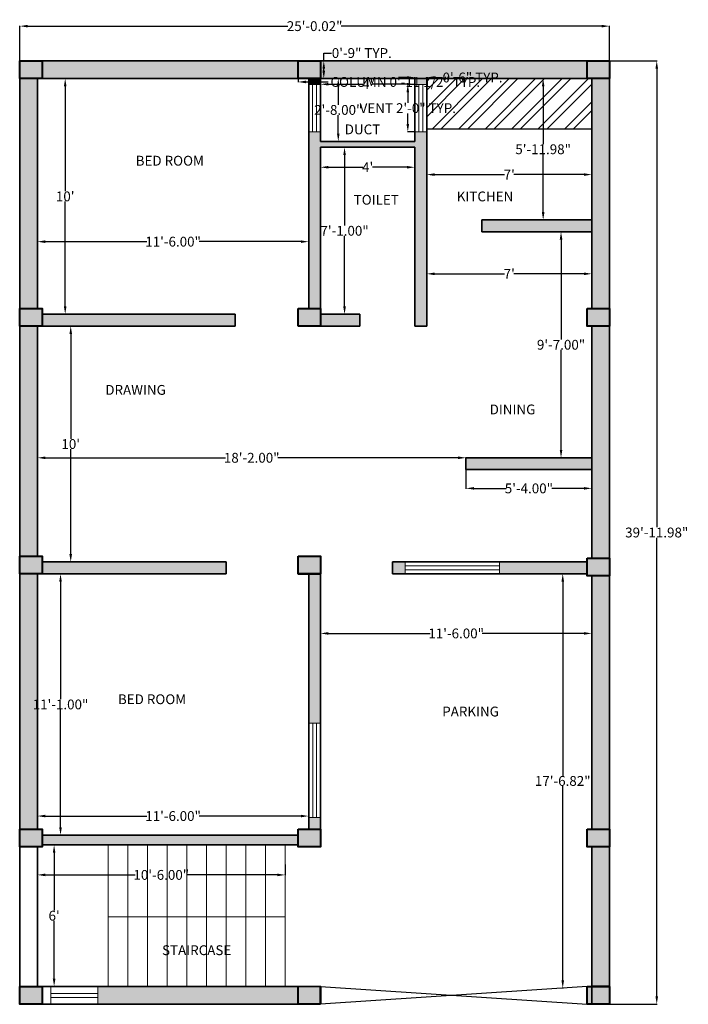
# Model space of a CAD drawing. Units: inches. Extents: x 107756 to 108945, y 133180 to 133782.
# Tile 1 of 3: x 107756 to 108096, y 133257 to 133758. Entities that reach past the tile are written whole.
import ezdxf

# ---------------------------------------------------------------- set-up
doc = ezdxf.new("R2010")
doc.units = ezdxf.units.IN
for name, color, linetype, lineweight in [('A-ANNO-DIMS', 2, 'Continuous', 13), ('A-AREA-IDEN', 7, 'Continuous', 18), ('A-CASE', 8, 'Continuous', 25), ('A-CASE-PATT', 8, 'Continuous', 13), ('A-COLS', 7, 'Continuous', 40), ('A-COLS-PATT', 6, 'Continuous', 13), ('A-DOOR', 3, 'Continuous', 25), ('A-FLOR-STRS', 7, 'Continuous', 18), ('A-GLAZ', 5, 'Continuous', 18), ('A-WALL', 7, 'Continuous', 35), ('A-WALL-PATT', 252, 'Continuous', 13)]:
    doc.layers.add(name, color=color, linetype=linetype, lineweight=lineweight)
doc.styles.get("Standard").update_dxf_attribs({"font": 'arial.ttf', "height": 5})
doc.dimstyles.get("Standard").update_dxf_attribs({"dimtxt": 5, "dimasz": 4, "dimexe": 0.18, "dimexo": 0.0625, "dimgap": 0.09, "dimtad": 0, "dimtih": 1, "dimtoh": 1, "dimzin": 0, "dimdsep": 46, "dimlunit": 3, "dimtxsty": 'Standard', "dimcen": 0.09, "dimclrd": 7, "dimclre": 256, "dimclrt": 256, "dimadec": 0, "dimazin": 0, "dimtfac": 1, "dimtofl": 0, "dimtmove": 0, "dimatfit": 3, "dimfxl": 1, "dimtolj": 1, "dimtzin": 0, "dimarcsym": 0})

# ---------------------------------------------------------------- blocks, each defined once
blk = doc.blocks.new('*D1')
at = {"layer": 'A-ANNO-DIMS', "color": 0, "lineweight": -2, "transparency": 16777216}
for p, q in [((107800.77, 133338.48), (107773.14, 133338.48)), ((107773.32, 133334.48), (107773.32, 133305.12)), ((107773.32, 133270.48), (107773.32, 133299.83)), ((107800.77, 133266.48), (107773.14, 133266.48))]:
    blk.add_line(p, q, dxfattribs=at)
at = {"layer": 'A-ANNO-DIMS', "color": 0, "transparency": 16777216}
for points in [[(107772.65, 133334.48), (107773.99, 133334.48), (107773.32, 133338.48)], [(107772.65, 133270.48), (107773.99, 133270.48), (107773.32, 133266.48)]]:
    blk.add_solid(points, dxfattribs=at)
at = {"layer": 'Defpoints', "color": 0, "transparency": 16777216}
for p in [(107773.32, 133338.48), (107800.84, 133338.48), (107800.84, 133266.48)]:
    blk.add_point(p, dxfattribs=at)
at = {"layer": 'A-ANNO-DIMS', "color": 0, "transparency": 16777216, "insert": (107773.32, 133302.48), "char_height": 5, "attachment_point": 5}
blk.add_mtext("\\A1;6'", dxfattribs=at)
blk = doc.blocks.new('*D2')
at = {"layer": 'A-ANNO-DIMS', "color": 0, "lineweight": -2, "transparency": 16777216}
for p, q in [((107764.84, 133328.53), (107764.84, 133323.07)), ((107890.84, 133328.53), (107890.84, 133323.07)), ((107768.84, 133323.25), (107814.54, 133323.25)), ((107886.84, 133323.25), (107841.13, 133323.25))]:
    blk.add_line(p, q, dxfattribs=at)
at = {"layer": 'A-ANNO-DIMS', "color": 0, "transparency": 16777216}
for points in [[(107768.84, 133323.92), (107768.84, 133322.58), (107764.84, 133323.25)], [(107886.84, 133323.92), (107886.84, 133322.58), (107890.84, 133323.25)]]:
    blk.add_solid(points, dxfattribs=at)
at = {"layer": 'Defpoints', "color": 0, "transparency": 16777216}
for p in [(107764.84, 133328.59), (107890.84, 133328.59), (107890.84, 133323.25)]:
    blk.add_point(p, dxfattribs=at)
at = {"layer": 'A-ANNO-DIMS', "color": 0, "transparency": 16777216, "insert": (107827.84, 133323.25), "char_height": 5, "attachment_point": 5}
blk.add_mtext('\\A1;10\'-6.00"', dxfattribs=at)
blk = doc.blocks.new('*D3')
at = {"layer": 'A-ANNO-DIMS', "color": 0, "lineweight": -2, "transparency": 16777216}
for p, q in [((107764.84, 133357.43), (107764.84, 133353.01)), ((107902.84, 133357.43), (107902.84, 133353.01)), ((107768.84, 133353.19), (107820.54, 133353.19)), ((107898.84, 133353.19), (107847.13, 133353.19))]:
    blk.add_line(p, q, dxfattribs=at)
at = {"layer": 'A-ANNO-DIMS', "color": 0, "transparency": 16777216}
for points in [[(107768.84, 133353.86), (107768.84, 133352.53), (107764.84, 133353.19)], [(107898.84, 133353.86), (107898.84, 133352.53), (107902.84, 133353.19)]]:
    blk.add_solid(points, dxfattribs=at)
at = {"layer": 'Defpoints', "color": 0, "transparency": 16777216}
for p in [(107764.84, 133357.49), (107902.84, 133357.49), (107902.84, 133353.19)]:
    blk.add_point(p, dxfattribs=at)
at = {"layer": 'A-ANNO-DIMS', "color": 0, "transparency": 16777216, "insert": (107833.84, 133353.19), "char_height": 5, "attachment_point": 5}
blk.add_mtext('\\A1;11\'-6.00"', dxfattribs=at)
blk = doc.blocks.new('*D4')
at = {"layer": 'A-ANNO-DIMS', "color": 0, "lineweight": -2, "transparency": 16777216}
for p, q in [((107791.72, 133476.48), (107776.4, 133476.48)), ((107776.58, 133472.48), (107776.58, 133412.62)), ((107776.58, 133347.48), (107776.58, 133407.33)), ((107791.72, 133343.48), (107776.4, 133343.48))]:
    blk.add_line(p, q, dxfattribs=at)
at = {"layer": 'A-ANNO-DIMS', "color": 0, "transparency": 16777216}
for points in [[(107775.91, 133472.48), (107777.24, 133472.48), (107776.58, 133476.48)], [(107775.91, 133347.48), (107777.24, 133347.48), (107776.58, 133343.48)]]:
    blk.add_solid(points, dxfattribs=at)
at = {"layer": 'Defpoints', "color": 0, "transparency": 16777216}
for p in [(107791.78, 133476.48), (107776.58, 133343.48), (107791.78, 133343.48)]:
    blk.add_point(p, dxfattribs=at)
at = {"layer": 'A-ANNO-DIMS', "color": 0, "transparency": 16777216, "insert": (107776.58, 133409.98), "char_height": 5, "attachment_point": 5}
blk.add_mtext('\\A1;11\'-1.00"', dxfattribs=at)
blk = doc.blocks.new('*D5')
at = {"layer": 'A-ANNO-DIMS', "color": 0, "lineweight": -2, "transparency": 16777216}
for p, q in [((107764.84, 133535.52), (107764.84, 133535.3)), ((107768.84, 133535.48), (107860.54, 133535.48)), ((107978.84, 133535.48), (107887.13, 133535.48)), ((107982.84, 133529.54), (107982.84, 133535.66))]:
    blk.add_line(p, q, dxfattribs=at)
at = {"layer": 'A-ANNO-DIMS', "color": 0, "transparency": 16777216}
for points in [[(107768.84, 133536.14), (107768.84, 133534.81), (107764.84, 133535.48)], [(107978.84, 133536.14), (107978.84, 133534.81), (107982.84, 133535.48)]]:
    blk.add_solid(points, dxfattribs=at)
at = {"layer": 'Defpoints', "color": 0, "transparency": 16777216}
for p in [(107764.84, 133535.58), (107982.84, 133535.48), (107982.84, 133529.48)]:
    blk.add_point(p, dxfattribs=at)
at = {"layer": 'A-ANNO-DIMS', "color": 0, "transparency": 16777216, "insert": (107873.84, 133535.48), "char_height": 5, "attachment_point": 5}
blk.add_mtext('\\A1;18\'-2.00"', dxfattribs=at)
blk = doc.blocks.new('*D6')
at = {"layer": 'A-ANNO-DIMS', "color": 0, "lineweight": -2, "transparency": 16777216}
for p, q in [((107775.93, 133602.48), (107781.95, 133602.48)), ((107781.77, 133598.48), (107781.77, 133545.12)), ((107781.77, 133486.48), (107781.77, 133539.83)), ((107775.93, 133482.48), (107781.95, 133482.48))]:
    blk.add_line(p, q, dxfattribs=at)
at = {"layer": 'A-ANNO-DIMS', "color": 0, "transparency": 16777216}
for points in [[(107781.11, 133598.48), (107782.44, 133598.48), (107781.77, 133602.48)], [(107781.11, 133486.48), (107782.44, 133486.48), (107781.77, 133482.48)]]:
    blk.add_solid(points, dxfattribs=at)
at = {"layer": 'Defpoints', "color": 0, "transparency": 16777216}
for p in [(107775.87, 133602.48), (107781.77, 133602.48), (107775.87, 133482.48)]:
    blk.add_point(p, dxfattribs=at)
at = {"layer": 'A-ANNO-DIMS', "color": 0, "transparency": 16777216, "insert": (107781.77, 133542.48), "char_height": 5, "attachment_point": 5}
blk.add_mtext("\\A1;10'", dxfattribs=at)
blk = doc.blocks.new('*D7')
at = {"layer": 'A-ANNO-DIMS', "color": 0, "lineweight": -2, "transparency": 16777216}
for p, q in [((107799.62, 133728.48), (107778.78, 133728.48)), ((107778.96, 133724.48), (107778.96, 133671.12)), ((107778.96, 133612.48), (107778.96, 133665.83)), ((107799.62, 133608.48), (107778.78, 133608.48))]:
    blk.add_line(p, q, dxfattribs=at)
at = {"layer": 'A-ANNO-DIMS', "color": 0, "transparency": 16777216}
for points in [[(107778.29, 133724.48), (107779.62, 133724.48), (107778.96, 133728.48)], [(107778.29, 133612.48), (107779.62, 133612.48), (107778.96, 133608.48)]]:
    blk.add_solid(points, dxfattribs=at)
at = {"layer": 'Defpoints', "color": 0, "transparency": 16777216}
for p in [(107778.96, 133728.48), (107799.68, 133728.48), (107799.68, 133608.48)]:
    blk.add_point(p, dxfattribs=at)
at = {"layer": 'A-ANNO-DIMS', "color": 0, "transparency": 16777216, "insert": (107778.96, 133668.48), "char_height": 5, "attachment_point": 5}
blk.add_mtext("\\A1;10'", dxfattribs=at)
blk = doc.blocks.new('*D8')
at = {"layer": 'A-ANNO-DIMS', "color": 0, "lineweight": -2, "transparency": 16777216}
for p, q in [((107764.84, 133651.21), (107764.84, 133645.27)), ((107902.84, 133651.21), (107902.84, 133645.27)), ((107768.84, 133645.45), (107820.54, 133645.45)), ((107898.84, 133645.45), (107847.13, 133645.45))]:
    blk.add_line(p, q, dxfattribs=at)
at = {"layer": 'A-ANNO-DIMS', "color": 0, "transparency": 16777216}
for points in [[(107768.84, 133646.11), (107768.84, 133644.78), (107764.84, 133645.45)], [(107898.84, 133646.11), (107898.84, 133644.78), (107902.84, 133645.45)]]:
    blk.add_solid(points, dxfattribs=at)
at = {"layer": 'Defpoints', "color": 0, "transparency": 16777216}
for p in [(107764.84, 133651.27), (107902.84, 133651.27), (107902.84, 133645.45)]:
    blk.add_point(p, dxfattribs=at)
at = {"layer": 'A-ANNO-DIMS', "color": 0, "transparency": 16777216, "insert": (107833.84, 133645.45), "char_height": 5, "attachment_point": 5}
blk.add_mtext('\\A1;11\'-6.00"', dxfattribs=at)
blk = doc.blocks.new('*D9')
at = {"layer": 'A-ANNO-DIMS', "color": 0, "lineweight": -2, "transparency": 16777216}
for p, q in [((107908.84, 133726.32), (107908.84, 133725.36)), ((107912.84, 133725.54), (107930.35, 133725.54)), ((107952.84, 133725.54), (107935.33, 133725.54)), ((107956.84, 133726.32), (107956.84, 133725.36))]:
    blk.add_line(p, q, dxfattribs=at)
at = {"layer": 'A-ANNO-DIMS', "color": 0, "transparency": 16777216}
for points in [[(107912.84, 133726.21), (107912.84, 133724.88), (107908.84, 133725.54)], [(107952.84, 133726.21), (107952.84, 133724.88), (107956.84, 133725.54)]]:
    blk.add_solid(points, dxfattribs=at)
at = {"layer": 'Defpoints', "color": 0, "transparency": 16777216}
for p in [(107908.84, 133726.38), (107956.84, 133726.38), (107956.84, 133725.54)]:
    blk.add_point(p, dxfattribs=at)
at = {"layer": 'A-ANNO-DIMS', "color": 0, "transparency": 16777216, "insert": (107932.84, 133725.54), "char_height": 5, "attachment_point": 5}
blk.add_mtext("\\A1;4'", dxfattribs=at)
blk = doc.blocks.new('*D10')
at = {"layer": 'A-ANNO-DIMS', "color": 0, "lineweight": -2, "transparency": 16777216}
for p, q in [((107914.64, 133728.48), (107918.05, 133728.48)), ((107917.87, 133724.48), (107917.87, 133715.12)), ((107917.87, 133700.48), (107917.87, 133709.83)), ((107914.64, 133696.48), (107918.05, 133696.48))]:
    blk.add_line(p, q, dxfattribs=at)
at = {"layer": 'A-ANNO-DIMS', "color": 0, "transparency": 16777216}
for points in [[(107917.2, 133724.48), (107918.54, 133724.48), (107917.87, 133728.48)], [(107917.2, 133700.48), (107918.54, 133700.48), (107917.87, 133696.48)]]:
    blk.add_solid(points, dxfattribs=at)
at = {"layer": 'Defpoints', "color": 0, "transparency": 16777216}
for p in [(107914.57, 133728.48), (107917.87, 133728.48), (107914.57, 133696.48)]:
    blk.add_point(p, dxfattribs=at)
at = {"layer": 'A-ANNO-DIMS', "color": 0, "transparency": 16777216, "insert": (107917.87, 133712.48), "char_height": 5, "attachment_point": 5}
blk.add_mtext('\\A1;2\'-8.00"', dxfattribs=at)
blk = doc.blocks.new('*D11')
at = {"layer": 'A-ANNO-DIMS', "color": 0, "lineweight": -2, "transparency": 16777216}
for p, q in [((107922.84, 133693.48), (107920.89, 133693.48)), ((107921.07, 133689.48), (107921.07, 133653.62)), ((107921.07, 133612.48), (107921.07, 133648.33)), ((107922.84, 133608.48), (107920.89, 133608.48))]:
    blk.add_line(p, q, dxfattribs=at)
at = {"layer": 'A-ANNO-DIMS', "color": 0, "transparency": 16777216}
for points in [[(107920.41, 133689.48), (107921.74, 133689.48), (107921.07, 133693.48)], [(107920.41, 133612.48), (107921.74, 133612.48), (107921.07, 133608.48)]]:
    blk.add_solid(points, dxfattribs=at)
at = {"layer": 'Defpoints', "color": 0, "transparency": 16777216}
for p in [(107921.07, 133693.48), (107922.9, 133693.48), (107922.9, 133608.48)]:
    blk.add_point(p, dxfattribs=at)
at = {"layer": 'A-ANNO-DIMS', "color": 0, "transparency": 16777216, "insert": (107921.07, 133650.98), "char_height": 5, "attachment_point": 5}
blk.add_mtext('\\A1;7\'-1.00"', dxfattribs=at)
blk = doc.blocks.new('*D12')
at = {"layer": 'A-ANNO-DIMS', "color": 0, "lineweight": -2, "transparency": 16777216}
for p, q in [((107908.84, 133693.41), (107908.84, 133683.14)), ((107956.84, 133693.41), (107956.84, 133683.14)), ((107912.84, 133683.32), (107930.35, 133683.32)), ((107952.84, 133683.32), (107935.33, 133683.32))]:
    blk.add_line(p, q, dxfattribs=at)
at = {"layer": 'A-ANNO-DIMS', "color": 0, "transparency": 16777216}
for points in [[(107912.84, 133683.98), (107912.84, 133682.65), (107908.84, 133683.32)], [(107952.84, 133683.98), (107952.84, 133682.65), (107956.84, 133683.32)]]:
    blk.add_solid(points, dxfattribs=at)
at = {"layer": 'Defpoints', "color": 0, "transparency": 16777216}
for p in [(107908.84, 133693.48), (107956.84, 133693.48), (107908.84, 133683.32)]:
    blk.add_point(p, dxfattribs=at)
at = {"layer": 'A-ANNO-DIMS', "color": 0, "transparency": 16777216, "insert": (107932.84, 133683.32), "char_height": 5, "attachment_point": 5}
blk.add_mtext("\\A1;4'", dxfattribs=at)
blk = doc.blocks.new('*D13')
at = {"layer": 'A-ANNO-DIMS', "color": 0, "lineweight": -2, "transparency": 16777216}
for p, q in [((108046.77, 133728.45), (108021.91, 133728.45)), ((108022.09, 133724.45), (108022.09, 133695.11)), ((108022.09, 133660.48), (108022.09, 133689.82)), ((108046.77, 133656.48), (108021.91, 133656.48))]:
    blk.add_line(p, q, dxfattribs=at)
at = {"layer": 'A-ANNO-DIMS', "color": 0, "transparency": 16777216}
for points in [[(108021.43, 133724.45), (108022.76, 133724.45), (108022.09, 133728.45)], [(108021.43, 133660.48), (108022.76, 133660.48), (108022.09, 133656.48)]]:
    blk.add_solid(points, dxfattribs=at)
at = {"layer": 'Defpoints', "color": 0, "transparency": 16777216}
for p in [(108022.09, 133728.45), (108046.84, 133728.45), (108046.84, 133656.48)]:
    blk.add_point(p, dxfattribs=at)
at = {"layer": 'A-ANNO-DIMS', "color": 0, "transparency": 16777216, "insert": (108022.09, 133692.46), "char_height": 5, "attachment_point": 5}
blk.add_mtext('\\A1;5\'-11.98"', dxfattribs=at)
blk = doc.blocks.new('*D14')
at = {"layer": 'A-ANNO-DIMS', "color": 0, "lineweight": -2, "transparency": 16777216}
for p, q in [((107962.84, 133691.71), (107962.84, 133679.39)), ((108046.84, 133691.71), (108046.84, 133679.39)), ((107966.84, 133679.57), (108002.47, 133679.57)), ((108042.84, 133679.57), (108007.21, 133679.57))]:
    blk.add_line(p, q, dxfattribs=at)
at = {"layer": 'A-ANNO-DIMS', "color": 0, "transparency": 16777216}
for points in [[(107966.84, 133680.24), (107966.84, 133678.91), (107962.84, 133679.57)], [(108042.84, 133680.24), (108042.84, 133678.91), (108046.84, 133679.57)]]:
    blk.add_solid(points, dxfattribs=at)
at = {"layer": 'Defpoints', "color": 0, "transparency": 16777216}
for p in [(107962.84, 133691.78), (108046.84, 133691.78), (108046.84, 133679.57)]:
    blk.add_point(p, dxfattribs=at)
at = {"layer": 'A-ANNO-DIMS', "color": 0, "transparency": 16777216, "insert": (108004.84, 133679.57), "char_height": 5, "attachment_point": 5}
blk.add_mtext("\\A1;7'", dxfattribs=at)
blk = doc.blocks.new('*D15')
at = {"layer": 'A-ANNO-DIMS', "color": 0, "lineweight": -2, "transparency": 16777216}
for p, q in [((107962.84, 133629.16), (107962.84, 133628.9)), ((107966.84, 133629.08), (108002.47, 133629.08)), ((108042.84, 133629.08), (108007.21, 133629.08)), ((108046.84, 133629.16), (108046.84, 133628.9))]:
    blk.add_line(p, q, dxfattribs=at)
at = {"layer": 'A-ANNO-DIMS', "color": 0, "transparency": 16777216}
for points in [[(107966.84, 133629.75), (107966.84, 133628.42), (107962.84, 133629.08)], [(108042.84, 133629.75), (108042.84, 133628.42), (108046.84, 133629.08)]]:
    blk.add_solid(points, dxfattribs=at)
at = {"layer": 'Defpoints', "color": 0, "transparency": 16777216}
for p in [(107962.84, 133629.23), (107962.84, 133629.08), (108046.84, 133629.23)]:
    blk.add_point(p, dxfattribs=at)
at = {"layer": 'A-ANNO-DIMS', "color": 0, "transparency": 16777216, "insert": (108004.84, 133629.08), "char_height": 5, "attachment_point": 5}
blk.add_mtext("\\A1;7'", dxfattribs=at)
blk = doc.blocks.new('*D16')
at = {"layer": 'A-ANNO-DIMS', "color": 0, "lineweight": -2, "transparency": 16777216}
for p, q in [((108037.82, 133650.48), (108031.01, 133650.48)), ((108031.19, 133646.48), (108031.19, 133595.62)), ((108031.19, 133539.48), (108031.19, 133590.33)), ((108037.82, 133535.48), (108031.01, 133535.48))]:
    blk.add_line(p, q, dxfattribs=at)
at = {"layer": 'A-ANNO-DIMS', "color": 0, "transparency": 16777216}
for points in [[(108030.53, 133646.48), (108031.86, 133646.48), (108031.19, 133650.48)], [(108030.53, 133539.48), (108031.86, 133539.48), (108031.19, 133535.48)]]:
    blk.add_solid(points, dxfattribs=at)
at = {"layer": 'Defpoints', "color": 0, "transparency": 16777216}
for p in [(108037.89, 133650.48), (108031.19, 133535.48), (108037.89, 133535.48)]:
    blk.add_point(p, dxfattribs=at)
at = {"layer": 'A-ANNO-DIMS', "color": 0, "transparency": 16777216, "insert": (108031.19, 133592.98), "char_height": 5, "attachment_point": 5}
blk.add_mtext('\\A1;9\'-7.00"', dxfattribs=at)
blk = doc.blocks.new('*D17')
at = {"layer": 'A-ANNO-DIMS', "color": 0, "lineweight": -2, "transparency": 16777216}
for p, q in [((107982.84, 133529.41), (107982.84, 133519.74)), ((108046.84, 133529.41), (108046.84, 133519.74)), ((107986.84, 133519.92), (108003.25, 133519.92)), ((108042.84, 133519.92), (108026.43, 133519.92))]:
    blk.add_line(p, q, dxfattribs=at)
at = {"layer": 'A-ANNO-DIMS', "color": 0, "transparency": 16777216}
for points in [[(107986.84, 133520.59), (107986.84, 133519.26), (107982.84, 133519.92)], [(108042.84, 133520.59), (108042.84, 133519.26), (108046.84, 133519.92)]]:
    blk.add_solid(points, dxfattribs=at)
at = {"layer": 'Defpoints', "color": 0, "transparency": 16777216}
for p in [(107982.84, 133529.48), (108046.84, 133529.48), (107982.84, 133519.92)]:
    blk.add_point(p, dxfattribs=at)
at = {"layer": 'A-ANNO-DIMS', "color": 0, "transparency": 16777216, "insert": (108014.84, 133519.92), "char_height": 5, "attachment_point": 5}
blk.add_mtext('\\A1;5\'-4.00"', dxfattribs=at)
blk = doc.blocks.new('*D18')
at = {"layer": 'A-ANNO-DIMS', "color": 0, "lineweight": -2, "transparency": 16777216}
for p, q in [((107908.84, 133439.92), (107908.84, 133446.29)), ((107912.84, 133446.11), (107964.54, 133446.11)), ((108042.84, 133446.11), (107991.13, 133446.11)), ((108046.84, 133439.92), (108046.84, 133446.29))]:
    blk.add_line(p, q, dxfattribs=at)
at = {"layer": 'A-ANNO-DIMS', "color": 0, "transparency": 16777216}
for points in [[(107912.84, 133446.78), (107912.84, 133445.45), (107908.84, 133446.11)], [(108042.84, 133446.78), (108042.84, 133445.45), (108046.84, 133446.11)]]:
    blk.add_solid(points, dxfattribs=at)
at = {"layer": 'Defpoints', "color": 0, "transparency": 16777216}
for p in [(107908.84, 133446.11), (107908.84, 133439.86), (108046.84, 133439.86)]:
    blk.add_point(p, dxfattribs=at)
at = {"layer": 'A-ANNO-DIMS', "color": 0, "transparency": 16777216, "insert": (107977.84, 133446.11), "char_height": 5, "attachment_point": 5}
blk.add_mtext('\\A1;11\'-6.00"', dxfattribs=at)
blk = doc.blocks.new('*D19')
at = {"layer": 'A-ANNO-DIMS', "color": 0, "lineweight": -2, "transparency": 16777216}
for p, q in [((108055.86, 133737.45), (108080.05, 133737.45)), ((108079.87, 133733.45), (108079.87, 133500.11)), ((108079.87, 133261.48), (108079.87, 133494.82)), ((108055.9, 133257.48), (108080.05, 133257.48))]:
    blk.add_line(p, q, dxfattribs=at)
at = {"layer": 'A-ANNO-DIMS', "color": 0, "transparency": 16777216}
for points in [[(108079.21, 133733.45), (108080.54, 133733.45), (108079.87, 133737.45)], [(108079.21, 133261.48), (108080.54, 133261.48), (108079.87, 133257.48)]]:
    blk.add_solid(points, dxfattribs=at)
at = {"layer": 'Defpoints', "color": 0, "transparency": 16777216}
for p in [(108055.8, 133737.45), (108055.84, 133257.48), (108079.87, 133257.48)]:
    blk.add_point(p, dxfattribs=at)
at = {"layer": 'A-ANNO-DIMS', "color": 0, "transparency": 16777216, "insert": (108079.87, 133497.46), "char_height": 5, "attachment_point": 5}
blk.add_mtext('\\A1;39\'-11.98"', dxfattribs=at)
blk = doc.blocks.new('*D20')
at = {"layer": 'A-ANNO-DIMS', "color": 0, "lineweight": -2, "transparency": 16777216}
for p, q in [((107755.84, 133737.54), (107755.84, 133755.29)), ((107759.84, 133755.11), (107892.27, 133755.11)), ((108051.86, 133755.11), (107919.42, 133755.11)), ((108055.86, 133737.51), (108055.86, 133755.29))]:
    blk.add_line(p, q, dxfattribs=at)
at = {"layer": 'A-ANNO-DIMS', "color": 0, "transparency": 16777216}
for points in [[(107759.84, 133755.77), (107759.84, 133754.44), (107755.84, 133755.11)], [(108051.86, 133755.77), (108051.86, 133754.44), (108055.86, 133755.11)]]:
    blk.add_solid(points, dxfattribs=at)
at = {"layer": 'Defpoints', "color": 0, "transparency": 16777216}
for p in [(108055.86, 133755.11), (107755.84, 133737.48), (108055.86, 133737.45)]:
    blk.add_point(p, dxfattribs=at)
at = {"layer": 'A-ANNO-DIMS', "color": 0, "transparency": 16777216, "insert": (107905.85, 133755.11), "char_height": 5, "attachment_point": 5}
blk.add_mtext('\\A1;25\'-0.02"', dxfattribs=at)
blk = doc.blocks.new('*D21')
at = {"layer": 'A-ANNO-DIMS', "color": 0, "lineweight": -2, "transparency": 16777216}
for p, q in [((108031.38, 133476.48), (108032.23, 133476.48)), ((108032.05, 133472.48), (108032.05, 133373.71)), ((108032.05, 133269.65), (108032.05, 133368.42)), ((108032.12, 133265.65), (108032.23, 133265.65))]:
    blk.add_line(p, q, dxfattribs=at)
at = {"layer": 'A-ANNO-DIMS', "color": 0, "transparency": 16777216}
for points in [[(108031.39, 133472.48), (108032.72, 133472.48), (108032.05, 133476.48)], [(108031.39, 133269.65), (108032.72, 133269.65), (108032.05, 133265.65)]]:
    blk.add_solid(points, dxfattribs=at)
at = {"layer": 'Defpoints', "color": 0, "transparency": 16777216}
for p in [(108031.32, 133476.48), (108032.05, 133265.65), (108032.05, 133265.65)]:
    blk.add_point(p, dxfattribs=at)
at = {"layer": 'A-ANNO-DIMS', "color": 0, "transparency": 16777216, "insert": (108032.05, 133371.06), "char_height": 5, "attachment_point": 5}
blk.add_mtext('\\A1;17\'-6.82"', dxfattribs=at)
blk = doc.blocks.new('WIN-VENT-24IN')
for p, q in [((0, 24), (6, 24)), ((2, 0), (2, 24)), ((4, 0), (4, 24)), ((0, 0), (6, 0))]:
    blk.add_line(p, q)
blk = doc.blocks.new('COL-RECT-11_37x9')
blk.add_lwpolyline([(0, 9), (11.37, 9), (11.37, 0), (0, 0)], close=True)
blk = doc.blocks.new('*D45')
at = {"layer": 'A-ANNO-DIMS', "lineweight": -2, "transparency": 16777216}
for p, q in [((107897.42, 133728.36), (107897.42, 133726.53)), ((107908.8, 133728.36), (107908.8, 133726.53))]:
    blk.add_line(p, q, dxfattribs=at)
at = {"layer": 'A-ANNO-DIMS', "color": 7, "lineweight": -2, "transparency": 16777216}
for p, q in [((107901.42, 133726.71), (107904.8, 133726.71)), ((107908.8, 133726.71), (107912.8, 133726.71))]:
    blk.add_line(p, q, dxfattribs=at)
at = {"layer": 'A-ANNO-DIMS', "color": 7, "transparency": 16777216}
for points in [[(107901.42, 133727.38), (107901.42, 133726.05), (107897.42, 133726.71)], [(107904.8, 133727.38), (107904.8, 133726.05), (107908.8, 133726.71)]]:
    blk.add_solid(points, dxfattribs=at)
at = {"layer": 'Defpoints', "color": 0, "transparency": 16777216}
for p in [(107897.42, 133728.42), (107908.8, 133728.42), (107908.8, 133726.71)]:
    blk.add_point(p, dxfattribs=at)
at = {"layer": 'A-ANNO-DIMS', "transparency": 16777216, "insert": (107951.97, 133726.71), "char_height": 5, "attachment_point": 5}
blk.add_mtext('\\A1;COLUMN 0\'-11 1/2" TYP.', dxfattribs=at)
blk = doc.blocks.new('*D46')
at = {"layer": 'A-ANNO-DIMS', "lineweight": -2, "transparency": 16777216}
for p, q in [((107908.86, 133737.42), (107910.68, 133737.42)), ((107908.86, 133728.42), (107910.68, 133728.42))]:
    blk.add_line(p, q, dxfattribs=at)
at = {"layer": 'A-ANNO-DIMS', "color": 7, "lineweight": -2, "transparency": 16777216}
for p, q in [((107910.5, 133737.42), (107910.5, 133741.42)), ((107910.5, 133741.42), (107914.5, 133741.42)), ((107910.5, 133732.42), (107910.5, 133733.42))]:
    blk.add_line(p, q, dxfattribs=at)
at = {"layer": 'A-ANNO-DIMS', "color": 7, "transparency": 16777216}
for points in [[(107909.83, 133733.42), (107911.17, 133733.42), (107910.5, 133737.42)], [(107909.83, 133732.42), (107911.17, 133732.42), (107910.5, 133728.42)]]:
    blk.add_solid(points, dxfattribs=at)
at = {"layer": 'Defpoints', "color": 0, "transparency": 16777216}
for p in [(107908.8, 133737.42), (107910.5, 133737.42), (107908.8, 133728.42)]:
    blk.add_point(p, dxfattribs=at)
at = {"layer": 'A-ANNO-DIMS', "transparency": 16777216, "insert": (107929.83, 133741.42), "char_height": 5, "attachment_point": 5}
blk.add_mtext('\\A1;0\'-9" TYP.', dxfattribs=at)
blk = doc.blocks.new('*D47')
at = {"layer": 'A-ANNO-DIMS', "lineweight": -2, "transparency": 16777216}
for p, q in [((107956.77, 133725.38), (107953.06, 133725.38)), ((107956.77, 133701.38), (107953.06, 133701.38))]:
    blk.add_line(p, q, dxfattribs=at)
at = {"layer": 'A-ANNO-DIMS', "color": 7, "lineweight": -2, "transparency": 16777216}
for p, q in [((107953.24, 133721.38), (107953.24, 133716.02)), ((107953.24, 133705.38), (107953.24, 133710.73))]:
    blk.add_line(p, q, dxfattribs=at)
at = {"layer": 'A-ANNO-DIMS', "color": 7, "transparency": 16777216}
for points in [[(107952.57, 133721.38), (107953.9, 133721.38), (107953.24, 133725.38)], [(107952.57, 133705.38), (107953.9, 133705.38), (107953.24, 133701.38)]]:
    blk.add_solid(points, dxfattribs=at)
at = {"layer": 'Defpoints', "color": 0, "transparency": 16777216}
for p in [(107953.24, 133725.38), (107956.84, 133725.38), (107956.84, 133701.38)]:
    blk.add_point(p, dxfattribs=at)
at = {"layer": 'A-ANNO-DIMS', "transparency": 16777216, "insert": (107953.24, 133713.38), "char_height": 5, "attachment_point": 5}
blk.add_mtext('\\A1;VENT 2\'-0" TYP.', dxfattribs=at)
blk = doc.blocks.new('*D48')
at = {"layer": 'A-ANNO-DIMS', "color": 7, "lineweight": -2, "transparency": 16777216}
for p, q in [((107952.84, 133728.98), (107948.84, 133728.98)), ((107966.84, 133728.98), (107970.84, 133728.98))]:
    blk.add_line(p, q, dxfattribs=at)
at = {"layer": 'A-ANNO-DIMS', "lineweight": -2, "transparency": 16777216}
for p, q in [((107956.84, 133725.44), (107956.84, 133729.16)), ((107962.84, 133725.44), (107962.84, 133729.16))]:
    blk.add_line(p, q, dxfattribs=at)
at = {"layer": 'A-ANNO-DIMS', "color": 7, "transparency": 16777216}
for points in [[(107952.84, 133729.64), (107952.84, 133728.31), (107956.84, 133728.98)], [(107966.84, 133729.64), (107966.84, 133728.31), (107962.84, 133728.98)]]:
    blk.add_solid(points, dxfattribs=at)
at = {"layer": 'Defpoints', "color": 0, "transparency": 16777216}
for p in [(107962.84, 133728.98), (107956.84, 133725.38), (107962.84, 133725.38)]:
    blk.add_point(p, dxfattribs=at)
at = {"layer": 'A-ANNO-DIMS', "transparency": 16777216, "insert": (107986.17, 133728.98), "char_height": 5, "attachment_point": 5}
blk.add_mtext('\\A1;0\'-6" TYP.', dxfattribs=at)

msp = doc.modelspace()

# ---------------------------------------------------------------- hatches: boundary and pattern name
at = {"layer": 'A-CASE-PATT'}
h = msp.add_hatch(dxfattribs=at)
h.set_pattern_fill('ANSI32', color=256)
h.set_pattern_definition([(45, (717.227, 52.435), (-6.7351921, 6.7351921), []), (45, (721.718, 52.435), (-6.7351921, 6.7351921), [])])
h.paths.add_polyline_path([(108046.837, 133702.908), (108046.837, 133728.452), (108044.427, 133728.452), (107962.837, 133728.459), (107962.837, 133702.908)])
at = {"layer": 'A-COLS-PATT'}
h = msp.add_hatch(color=256, dxfattribs=at)
h.dxf.hatch_style = 1
h.paths.add_polyline_path([(107767.208, 133485.477), (107755.837, 133485.477), (107755.837, 133476.477), (107767.208, 133476.477)])
h.paths.add_polyline_path([(107908.837, 133485.477), (107897.467, 133485.477), (107897.467, 133476.477), (107908.837, 133476.477)])
h.paths.add_polyline_path([(107908.837, 133346.477), (107897.467, 133346.477), (107897.467, 133337.477), (107908.837, 133337.477)])
h.paths.add_polyline_path([(107767.208, 133346.477), (107755.837, 133346.477), (107755.837, 133337.477), (107767.208, 133337.477)])
h.paths.add_polyline_path([(107767.208, 133266.477), (107755.837, 133266.477), (107755.837, 133257.477), (107767.208, 133257.477)])
h.paths.add_polyline_path([(107908.837, 133266.477), (107897.467, 133266.477), (107897.467, 133257.477), (107908.837, 133257.477)])
h.paths.add_polyline_path([(108055.837, 133266.477), (108046.837, 133266.477), (108046.837, 133257.477), (108055.837, 133257.477)])
h.paths.add_polyline_path([(108046.837, 133266.477), (108044.467, 133266.477), (108044.467, 133257.477), (108046.837, 133257.477)])
h.paths.add_polyline_path([(108055.837, 133346.477), (108044.467, 133346.477), (108044.467, 133337.477), (108055.837, 133337.477)])
h.paths.add_polyline_path([(108055.837, 133484.477), (108044.467, 133484.477), (108044.467, 133475.477), (108055.837, 133475.477)])
h.paths.add_polyline_path([(108055.837, 133611.477), (108044.467, 133611.477), (108044.467, 133602.477), (108055.837, 133602.477)])
h.paths.add_polyline_path([(108055.798, 133737.452), (108044.427, 133737.452), (108044.427, 133728.477), (108046.837, 133728.477), (108055.798, 133728.452)])
h.paths.add_polyline_path([(107767.208, 133737.477), (107755.837, 133737.477), (107755.837, 133728.477), (107767.208, 133728.477)])
h.paths.add_polyline_path([(107908.795, 133737.42), (107897.425, 133737.42), (107897.425, 133728.477), (107908.795, 133728.477)])
h.paths.add_polyline_path([(107908.837, 133611.477), (107897.467, 133611.477), (107897.467, 133602.477), (107908.837, 133602.477)])
h.paths.add_polyline_path([(107767.184, 133611.478), (107755.837, 133611.478), (107755.837, 133602.478), (107767.184, 133602.478)])
at = {"layer": 'A-WALL-PATT'}
h = msp.add_hatch(color=256, dxfattribs=at)
h.dxf.hatch_style = 1
h.paths.add_polyline_path([(107764.837, 133476.477), (107755.837, 133476.477), (107755.837, 133346.477), (107764.837, 133346.477)])
h.paths.add_polyline_path([(107860.893, 133476.477), (107860.893, 133482.477), (107767.208, 133482.477), (107767.208, 133476.477)])
h.paths.add_polyline_path([(107897.467, 133338.477), (107897.467, 133343.477), (107767.208, 133343.477), (107767.208, 133338.477)])
h.paths.add_polyline_path([(107908.837, 133476.477), (107902.837, 133476.477), (107902.837, 133400.531), (107908.837, 133400.531)])
h.paths.add_polyline_path([(107908.837, 133346.477), (107908.837, 133352.531), (107902.837, 133352.531), (107902.837, 133346.477)])
h.paths.add_polyline_path([(107999.961, 133482.477), (107999.961, 133476.477), (108044.467, 133476.477), (108044.467, 133482.477)])
h.paths.add_polyline_path([(107945.411, 133482.477), (107945.411, 133476.477), (107951.961, 133476.477), (107951.961, 133482.477)])
h.paths.add_polyline_path([(107982.837, 133535.477), (107982.837, 133529.477), (108046.837, 133529.477), (108046.837, 133535.477)])
h.paths.add_polyline_path([(108046.837, 133529.477), (108046.837, 133484.477), (108055.837, 133484.477), (108055.837, 133602.477), (108046.837, 133602.477)])
h.paths.add_polyline_path([(108055.837, 133475.477), (108046.837, 133475.477), (108046.837, 133346.477), (108055.837, 133346.477)])
h.paths.add_polyline_path([(108055.837, 133337.477), (108046.837, 133337.477), (108046.837, 133266.477), (108055.837, 133266.477)])
h.paths.add_polyline_path([(108046.837, 133611.477), (108055.837, 133611.477), (108055.837, 133728.452), (108046.837, 133728.452)])
h.paths.add_polyline_path([(107956.837, 133608.477), (107956.837, 133602.477), (107962.837, 133602.477), (107962.837, 133701.376), (107956.837, 133701.376), (107956.837, 133696.477), (107908.837, 133696.477), (107908.837, 133701.376), (107902.837, 133701.376), (107902.837, 133611.477), (107908.837, 133611.477), (107908.837, 133693.477), (107956.837, 133693.477)])
h.paths.add_polyline_path([(107962.837, 133725.376), (107962.837, 133728.477), (107956.837, 133728.477), (107956.837, 133725.376)])
h.paths.add_polyline_path([(108044.427, 133728.477), (108044.427, 133737.477), (107908.837, 133737.477), (107908.837, 133728.477)])
h.paths.add_polyline_path([(107767.208, 133737.477), (107767.208, 133728.477), (107897.425, 133728.477), (107897.425, 133737.477)])
h.paths.add_polyline_path([(107764.837, 133728.477), (107755.837, 133728.477), (107755.837, 133611.478), (107764.837, 133611.478)])
h.paths.add_polyline_path([(107755.837, 133485.477), (107764.837, 133485.477), (107764.837, 133602.478), (107755.837, 133602.478)])
h.paths.add_polyline_path([(107795.626, 133266.477), (107795.626, 133257.477), (107897.467, 133257.477), (107897.467, 133266.477)])
h = msp.add_hatch(color=256, dxfattribs=at)
h.dxf.hatch_style = 1
h.paths.add_polyline_path([(107902.837, 133728.42), (107902.837, 133725.376), (107908.837, 133725.376), (107908.837, 133728.42)])
h = msp.add_hatch(color=256, dxfattribs=at)
h.dxf.hatch_style = 1
h.paths.add_polyline_path([(108046.837, 133650.477), (108046.837, 133656.477), (107990.837, 133656.477), (107990.837, 133650.477)])
h = msp.add_hatch(color=256, dxfattribs=at)
h.dxf.hatch_style = 1
h.paths.add_polyline_path([(107865.467, 133608.477), (107767.184, 133608.477), (107767.184, 133602.477), (107865.467, 133602.477)])
h.paths.add_polyline_path([(107908.837, 133608.477), (107908.837, 133602.477), (107928.837, 133602.477), (107928.837, 133608.477)])

# ---------------------------------------------------------------- linework, layer by layer
at = {"layer": 'A-CASE'}
msp.add_line((107962.837, 133702.908), (108046.837, 133702.908), dxfattribs=at)
at = {"layer": 'A-COLS'}
for p, q in [((107897.467, 133611.477), (107908.837, 133611.477)), ((107897.467, 133602.477), (107897.467, 133611.477)), ((107908.837, 133611.477), (107908.837, 133602.477)), ((107908.837, 133602.477), (107897.467, 133602.477)), ((107897.467, 133476.477), (107908.837, 133476.477)), ((107897.467, 133257.477), (107897.467, 133266.477)), ((107908.837, 133266.477), (107908.837, 133257.477)), ((107908.837, 133257.477), (107897.467, 133257.477))]:
    msp.add_line(p, q, dxfattribs=at)
msp.add_lwpolyline([(107908.837, 133257.477), (107908.837, 133257.477), (107908.837, 133266.477), (107908.837, 133266.477)], close=True, dxfattribs=at)
msp.add_lwpolyline([(107908.837, 133257.477), (107908.837, 133257.477), (107908.837, 133266.477), (107908.837, 133266.477)], close=True, dxfattribs=at)
for points in [[(108055.837, 133266.477), (108046.837, 133266.477)], [(108055.837, 133257.477), (108046.837, 133257.477)]]:
    msp.add_lwpolyline(points, dxfattribs=at)
at = {"layer": 'A-DOOR'}
for p, q in [((107908.837, 133266.477), (108044.467, 133257.477)), ((108044.467, 133266.477), (107908.837, 133257.477))]:
    msp.add_line(p, q, dxfattribs=at)
at = {"layer": 'A-FLOR-STRS'}
for p, q in [((107800.837, 133266.477), (107800.837, 133338.477)), ((107810.837, 133266.477), (107810.837, 133338.477)), ((107820.837, 133266.477), (107820.837, 133338.477)), ((107830.837, 133266.477), (107830.837, 133338.477)), ((107840.837, 133266.477), (107840.837, 133338.477)), ((107850.837, 133266.477), (107850.837, 133338.477)), ((107860.837, 133266.477), (107860.837, 133338.477)), ((107870.837, 133266.477), (107870.837, 133338.477)), ((107880.837, 133266.477), (107880.837, 133338.477)), ((107890.837, 133266.477), (107890.837, 133338.477)), ((107800.837, 133301.977), (107890.837, 133301.977))]:
    msp.add_line(p, q, dxfattribs=at)
at = {"layer": 'A-GLAZ'}
for p, q in [((107951.961, 133482.477), (107951.961, 133476.477)), ((107999.961, 133482.477), (107999.961, 133476.477)), ((107999.961, 133480.477), (107951.961, 133480.477)), ((107999.961, 133478.477), (107951.961, 133478.477)), ((107908.87, 133400.531), (107902.837, 133400.531)), ((107904.854, 133352.531), (107904.854, 133400.531)), ((107906.854, 133352.531), (107906.854, 133400.531)), ((107908.87, 133352.531), (107902.837, 133352.531)), ((107771.626, 133257.405), (107771.626, 133266.376)), ((107795.626, 133257.405), (107795.626, 133266.376)), ((107795.626, 133262.891), (107771.626, 133262.891)), ((107795.626, 133260.891), (107771.626, 133260.891))]:
    msp.add_line(p, q, dxfattribs=at)
at = {"layer": 'A-WALL'}
for p, q in [((107908.837, 133696.477), (107908.837, 133737.477)), ((107764.837, 133728.477), (108046.837, 133728.477)), ((107764.837, 133611.478), (107764.837, 133728.477)), ((107902.837, 133611.477), (107902.837, 133728.477)), ((107956.837, 133728.477), (107956.837, 133696.477)), ((107962.837, 133728.477), (107962.837, 133602.477)), ((108046.837, 133728.477), (108046.837, 133611.477)), ((107908.837, 133696.477), (107956.837, 133696.477)), ((107908.837, 133693.477), (107956.837, 133693.477)), ((107908.837, 133602.477), (107908.837, 133693.477)), ((107956.837, 133693.477), (107956.837, 133608.477)), ((107990.837, 133656.477), (108046.837, 133656.477)), ((107990.837, 133656.477), (107990.837, 133650.477)), ((107990.837, 133650.477), (108046.837, 133650.477)), ((107767.184, 133608.477), (107865.467, 133608.477)), ((107865.467, 133602.477), (107865.467, 133608.477)), ((107908.837, 133608.477), (107928.837, 133608.477)), ((107928.837, 133608.477), (107928.837, 133602.477)), ((107956.837, 133608.477), (107956.837, 133602.477)), ((107764.837, 133485.477), (107764.837, 133602.478)), ((107764.837, 133602.477), (107865.467, 133602.477)), ((107897.467, 133602.477), (107928.837, 133602.477)), ((107956.837, 133602.477), (107962.837, 133602.477)), ((108046.837, 133602.477), (108046.837, 133529.477)), ((107982.837, 133535.477), (108046.837, 133535.477)), ((107982.837, 133529.477), (107982.837, 133535.477)), ((107982.837, 133529.477), (108046.837, 133529.477)), ((108046.837, 133529.477), (108046.837, 133506.477)), ((108046.837, 133529.477), (108046.837, 133484.477)), ((107767.208, 133482.477), (107860.893, 133482.477)), ((107860.893, 133476.477), (107860.893, 133482.477)), ((107908.837, 133337.477), (107908.837, 133482.477)), ((107945.411, 133482.477), (108044.467, 133482.477)), ((107945.411, 133476.477), (107945.411, 133482.477)), ((107764.837, 133476.477), (107860.893, 133476.477)), ((107902.837, 133346.477), (107902.837, 133476.477)), ((107945.411, 133476.477), (108044.467, 133476.477)), ((108046.837, 133475.477), (108046.837, 133346.477)), ((107767.208, 133343.477), (107897.467, 133343.477)), ((107764.837, 133266.477), (107764.837, 133337.477)), ((107767.208, 133338.477), (107897.467, 133338.477)), ((108046.837, 133337.477), (108046.837, 133257.477)), ((107908.837, 133266.477), (107764.837, 133266.477)), ((107908.837, 133257.477), (107908.837, 133266.477))]:
    msp.add_line(p, q, dxfattribs=at)
for points in [[(107755.837, 133476.477), (107755.837, 133737.477), (108055.837, 133737.477), (108055.837, 133257.477)], [(107755.837, 133346.477), (107755.837, 133476.477)], [(107764.837, 133346.477), (107764.837, 133476.477)], [(107908.837, 133257.477), (107755.837, 133257.477), (107755.837, 133346.477)]]:
    msp.add_lwpolyline(points, dxfattribs=at)

# ---------------------------------------------------------------- block references
at = {"layer": 'A-COLS'}
for p in [(107755.837, 133728.477), (107897.425, 133728.42), (108044.427, 133728.452), (107755.813, 133602.478), (108044.467, 133602.477), (107755.837, 133476.477), (107897.467, 133476.477), (108044.467, 133475.477), (107755.837, 133337.477), (107897.467, 133337.477), (108044.467, 133337.477), (107755.837, 133257.477), (108044.467, 133257.477)]:
    msp.add_blockref('COL-RECT-11_37x9', p, dxfattribs=at)
at = {"layer": 'A-GLAZ'}
for p in [(107902.837, 133701.376), (107956.837, 133701.376)]:
    msp.add_blockref('WIN-VENT-24IN', p, dxfattribs=at)

# ---------------------------------------------------------------- texts
at = {"layer": 'A-AREA-IDEN', "char_height": 5, "attachment_point": 1}
for s, width, insert in [('DUCT', 30.72767, (107921.166, 133705.068)), ('BED ROOM ', 38.58355, (107814.812, 133689.131)), ('TOILET', 24.50297, (107925.711, 133669.273)), ('\\pxqc;KITCHEN', 50.06099, (107967.498, 133670.955)), ('DRAWING', 36.26073, (107799.358, 133572.519)), ('\\pxqc;DINING', 38.2328, (107987.385, 133562.577)), ('BED ROOM ', 38.58355, (107805.776, 133415.12)), ('PARKING', 37.58343, (107970.755, 133408.859)), ('\\pxqc;STAIRCASE', 70, (107810.837, 133287.435))]:
    msp.add_mtext_dynamic_manual_height_columns(s, width=width, gutter_width=25, heights=[0], dxfattribs=dict(at, insert=insert))

# ---------------------------------------------------------------- dimensions: what is measured, and where the dimension line sits
at = {"layer": 'A-ANNO-DIMS'}
for base, p1, p2, picture, middle in [((108055.86, 133755.106), (107755.837, 133737.477), (108055.86, 133737.452), '*D20', (107905.849, 133755.106)), ((107956.837, 133725.545), (107908.837, 133726.383), (107956.837, 133726.383), '*D9', (107932.837, 133725.545)), ((107908.837, 133683.317), (107956.837, 133693.477), (107908.837, 133693.477), '*D12', (107932.837, 133683.317)), ((108046.837, 133679.573), (107962.837, 133691.777), (108046.837, 133691.777), '*D14', (108004.837, 133679.573)), ((107902.837, 133645.446), (107764.837, 133651.269), (107902.837, 133651.269), '*D8', (107833.837, 133645.446)), ((107962.837, 133629.084), (108046.837, 133629.227), (107962.837, 133629.227), '*D15', (108004.837, 133629.084)), ((107982.837, 133535.477), (107764.837, 133535.583), (107982.837, 133529.477), '*D5', (107873.837, 133535.477)), ((107982.837, 133519.922), (108046.837, 133529.477), (107982.837, 133529.477), '*D17', (108014.837, 133519.922)), ((107908.837, 133446.114), (108046.837, 133439.859), (107908.837, 133439.859), '*D18', (107977.837, 133446.114)), ((107902.837, 133353.193), (107764.837, 133357.491), (107902.837, 133357.491), '*D3', (107833.837, 133353.193)), ((107890.837, 133323.251), (107764.837, 133328.59), (107890.837, 133328.59), '*D2', (107827.837, 133323.251))]:
    dim = msp.add_linear_dim(base=base, p1=p1, p2=p2, dimstyle='Standard', override={"dimclrd": 0, "dimclre": 0, "dimclrt": 0}, dxfattribs=at)
    dim.commit()
    dim.dimension.update_dxf_attribs({"geometry": picture, "text_midpoint": middle})
for base, p1, p2, text, picture, middle in [((107910.501, 133737.42), (107908.795, 133728.42), (107908.795, 133737.42), '<> TYP.', '*D46', (107929.83, 133741.42)), ((107953.237, 133725.376), (107956.837, 133701.376), (107956.837, 133725.376), 'VENT <> TYP.', '*D47', (107953.237, 133713.376))]:
    dim = msp.add_linear_dim(base=base, p1=p1, p2=p2, angle=90, text=text, dimstyle='Standard', override={"dimdec": 1, "dimlfac": 1, "dimrnd": 0, "dimzin": 1, "dimdsep": 46, "dimlunit": 4, "dimfrac": 2}, dxfattribs=at)
    dim.commit()
    dim.dimension.update_dxf_attribs({"geometry": picture, "text_midpoint": middle})
for base, p1, p2, text, picture, middle in [((107908.795, 133726.714), (107897.425, 133728.42), (107908.795, 133728.42), 'COLUMN <> TYP.', '*D45', (107951.968, 133726.714)), ((107962.837, 133728.976), (107956.837, 133725.376), (107962.837, 133725.376), '<> TYP.', '*D48', (107986.166, 133728.976))]:
    dim = msp.add_linear_dim(base=base, p1=p1, p2=p2, text=text, dimstyle='Standard', override={"dimdec": 1, "dimlfac": 1, "dimrnd": 0, "dimzin": 1, "dimdsep": 46, "dimlunit": 4, "dimfrac": 2}, dxfattribs=at)
    dim.commit()
    dim.dimension.update_dxf_attribs({"geometry": picture, "text_midpoint": middle})
for base, p1, p2, picture, middle in [((108079.8723, 133257.4766), (108055.7975, 133737.4518), (108055.8373, 133257.4766), '*D19', (108079.8723, 133497.4642)), ((107778.957, 133728.477), (107799.679, 133608.477), (107799.679, 133728.477), '*D7', (107778.957, 133668.477)), ((107917.87, 133728.477), (107914.573, 133696.477), (107914.573, 133728.477), '*D10', (107917.87, 133712.477)), ((108022.0949, 133728.4518), (108046.8373, 133656.4766), (108046.8373, 133728.4518), '*D13', (108022.0949, 133692.4642)), ((107921.074, 133693.477), (107922.904, 133608.477), (107922.904, 133693.477), '*D11', (107921.074, 133650.977)), ((108031.192, 133535.477), (108037.886, 133650.477), (108037.886, 133535.477), '*D16', (108031.192, 133592.977)), ((107781.774, 133602.477), (107775.871, 133482.477), (107775.871, 133602.477), '*D6', (107781.774, 133542.477)), ((107776.576, 133343.477), (107791.781, 133476.477), (107791.781, 133343.477), '*D4', (107776.576, 133409.977)), ((108032.054, 133265.653), (108031.321, 133476.477), (108032.054, 133265.653), '*D21', (108032.054, 133371.065)), ((107773.32, 133338.477), (107800.837, 133266.477), (107800.837, 133338.477), '*D1', (107773.32, 133302.477))]:
    dim = msp.add_linear_dim(base=base, p1=p1, p2=p2, angle=90, dimstyle='Standard', override={"dimclrd": 0, "dimclre": 0, "dimclrt": 0}, dxfattribs=at)
    dim.commit()
    dim.dimension.update_dxf_attribs({"geometry": picture, "text_midpoint": middle})

doc.saveas('drawing.dxf')
